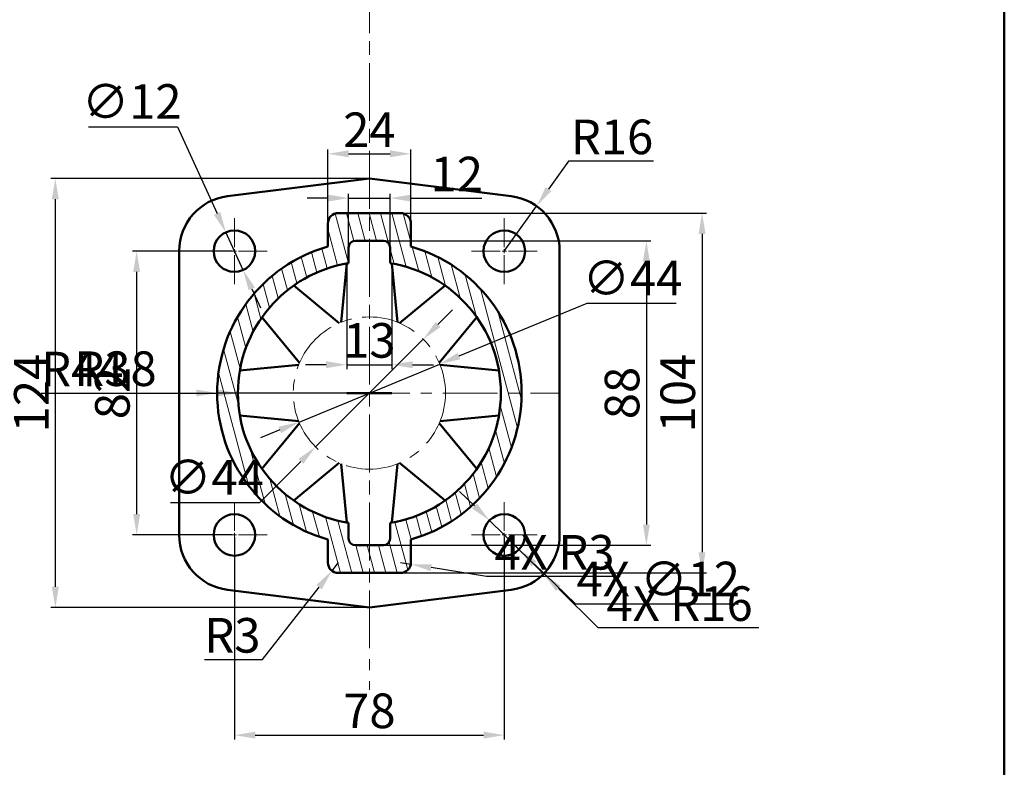
# Model space of a CAD drawing. Units: millimetres. Extents: x 147 to 984, y -369 to 435.
# Tile 9 of 10: x 699 to 984, y -34 to 182. Entities that reach past the tile are written whole.
import ezdxf

# ---------------------------------------------------------------- set-up
doc = ezdxf.new("R2010")
doc.units = ezdxf.units.MM
doc.header["$LTSCALE"] = 0.5
doc.linetypes.add('CENTER', pattern=[50.8, 31.75, -6.35, 6.35, -6.35])
for name, color, linetype, lineweight in [('M-CNTR', 1, 'CENTER', 18), ('M-DIMS', 2, 'Continuous', 25), ('M-HATC', 8, 'Continuous', 18), ('M-OUTL', 7, 'Continuous', 50)]:
    doc.layers.add(name, color=color, linetype=linetype, lineweight=lineweight)
doc.styles.get("Standard").update_dxf_attribs({"font": 'arial.ttf'})
doc.dimstyles.new('ISO-25', dxfattribs={"dimtxt": 10, "dimasz": 6, "dimexe": 1.25, "dimexo": 0.625, "dimtad": 1, "dimtoh": 1, "dimdec": 0, "dimtxsty": 'Standard', "dimcen": 2.5, "dimadec": 0, "dimazin": 0, "dimtfac": 1, "dimtdec": 0, "dimtmove": 0, "dimatfit": 3, "dimfxl": 1, "dimarcsym": 0})

# ---------------------------------------------------------------- blocks, each defined once
blk = doc.blocks.new('*U58')
at = {"layer": 'M-CNTR', "color": 0, "transparency": 16777216}
for p, q in [((0, 1.2), (0, 9.5)), ((-9.5, 0), (-1.2, 0)), ((1.2, 0), (9.5, 0)), ((0, -9.5), (0, -1.2))]:
    blk.add_line(p, q, dxfattribs=at)
at = {"layer": 'M-CNTR', "color": 0, "linetype": 'Continuous', "transparency": 16777216}
for p, q in [((-0.6, 0), (0.6, 0)), ((0, -0.6), (0, 0.6))]:
    blk.add_line(p, q, dxfattribs=at)
blk = doc.blocks.new('*U59')
at = {"layer": 'M-CNTR', "color": 0, "transparency": 16777216}
for p, q in [((0, 1.2), (0, 9.5)), ((-9.5, 0), (-1.2, 0)), ((1.2, 0), (9.5, 0)), ((0, -9.5), (0, -1.2))]:
    blk.add_line(p, q, dxfattribs=at)
at = {"layer": 'M-CNTR', "color": 0, "linetype": 'Continuous', "transparency": 16777216}
for p, q in [((-0.6, 0), (0.6, 0)), ((0, -0.6), (0, 0.6))]:
    blk.add_line(p, q, dxfattribs=at)
blk = doc.blocks.new('*U60')
at = {"layer": 'M-CNTR', "color": 0, "transparency": 16777216}
for p, q in [((0, 1.2), (0, 9.5)), ((-9.5, 0), (-1.2, 0)), ((1.2, 0), (9.5, 0)), ((0, -9.5), (0, -1.2))]:
    blk.add_line(p, q, dxfattribs=at)
at = {"layer": 'M-CNTR', "color": 0, "linetype": 'Continuous', "transparency": 16777216}
for p, q in [((-0.6, 0), (0.6, 0)), ((0, -0.6), (0, 0.6))]:
    blk.add_line(p, q, dxfattribs=at)
blk = doc.blocks.new('*U61')
at = {"layer": 'M-CNTR', "color": 0, "transparency": 16777216}
for p, q in [((0, 1.2), (0, 9.5)), ((-9.5, 0), (-1.2, 0)), ((1.2, 0), (9.5, 0)), ((0, -9.5), (0, -1.2))]:
    blk.add_line(p, q, dxfattribs=at)
at = {"layer": 'M-CNTR', "color": 0, "linetype": 'Continuous', "transparency": 16777216}
for p, q in [((-0.6, 0), (0.6, 0)), ((0, -0.6), (0, 0.6))]:
    blk.add_line(p, q, dxfattribs=at)
blk = doc.blocks.new('*U62')
at = {"layer": 'M-CNTR', "color": 0, "transparency": 16777216}
blk.add_line((0, 99.41), (0, -106.28), dxfattribs=at)
blk = doc.blocks.new('*D63')
at = {"layer": 'Defpoints', "color": 0, "transparency": 16777216}
for p in [(800.56, 136.03), (709.78, 12.03), (800.56, 12.03)]:
    blk.add_point(p, dxfattribs=at)
at = {"layer": 'M-DIMS', "color": 0, "lineweight": -2, "transparency": 16777216}
for p, q in [((799.93, 136.03), (708.53, 136.03)), ((709.78, 130.03), (709.78, 18.03)), ((799.93, 12.03), (708.53, 12.03))]:
    blk.add_line(p, q, dxfattribs=at)
at = {"layer": 'M-DIMS', "color": 0, "transparency": 16777216}
for points in [[(708.78, 130.03), (710.78, 130.03), (709.78, 136.03)], [(708.78, 18.03), (710.78, 18.03), (709.78, 12.03)]]:
    blk.add_solid(points, dxfattribs=at)
at = {"layer": 'M-DIMS', "color": 0, "transparency": 16777216, "insert": (704.14, 74.03), "char_height": 10, "attachment_point": 5, "rotation": 90}
blk.add_mtext('124', dxfattribs=at)
blk = doc.blocks.new('*D64')
at = {"layer": 'Defpoints', "color": 0, "transparency": 16777216}
for p in [(761.56, 115.03), (733.29, 33.03), (761.56, 33.03)]:
    blk.add_point(p, dxfattribs=at)
at = {"layer": 'M-DIMS', "color": 0, "lineweight": -2, "transparency": 16777216}
for p, q in [((760.93, 115.03), (732.04, 115.03)), ((733.29, 109.03), (733.29, 39.03)), ((760.93, 33.03), (732.04, 33.03))]:
    blk.add_line(p, q, dxfattribs=at)
at = {"layer": 'M-DIMS', "color": 0, "transparency": 16777216}
for points in [[(732.29, 109.03), (734.29, 109.03), (733.29, 115.03)], [(732.29, 39.03), (734.29, 39.03), (733.29, 33.03)]]:
    blk.add_solid(points, dxfattribs=at)
at = {"layer": 'M-DIMS', "color": 0, "transparency": 16777216, "insert": (727.56, 74.03), "char_height": 10, "attachment_point": 5, "rotation": 90}
blk.add_mtext('82', dxfattribs=at)
blk = doc.blocks.new('*D65')
at = {"layer": 'Defpoints', "color": 0, "transparency": 16777216}
for p in [(759.05, 120.48), (764.06, 109.58)]:
    blk.add_point(p, dxfattribs=at)
at = {"layer": 'M-DIMS', "color": 0, "lineweight": -2, "transparency": 16777216}
for p, q in [((719.33, 150.97), (745.06, 150.97)), ((745.06, 150.97), (756.55, 125.93)), ((764.06, 109.58), (759.05, 120.48)), ((766.56, 104.12), (769.07, 98.67))]:
    blk.add_line(p, q, dxfattribs=at)
at = {"layer": 'M-DIMS', "color": 0, "transparency": 16777216}
for points in [[(757.46, 126.35), (755.64, 125.52), (759.05, 120.48)], [(767.47, 104.54), (765.66, 103.7), (764.06, 109.58)]]:
    blk.add_solid(points, dxfattribs=at)
at = {"layer": 'M-DIMS', "color": 0, "transparency": 16777216, "insert": (731.88, 156.98), "char_height": 10, "attachment_point": 5}
blk.add_mtext('∅12', dxfattribs=at)
blk = doc.blocks.new('*D66')
at = {"layer": 'Defpoints', "color": 0, "transparency": 16777216}
for p in [(848.86, 128.04), (839.56, 115.03)]:
    blk.add_point(p, dxfattribs=at)
at = {"layer": 'M-DIMS', "color": 0, "lineweight": -2, "transparency": 16777216}
for p, q in [((858.14, 141.02), (852.35, 132.92)), ((882.65, 141.02), (858.14, 141.02)), ((839.56, 115.03), (848.86, 128.04))]:
    blk.add_line(p, q, dxfattribs=at)
at = {"layer": 'M-DIMS', "color": 0, "transparency": 16777216}
blk.add_solid([(851.54, 133.51), (853.17, 132.34), (848.86, 128.04)], dxfattribs=at)
at = {"layer": 'M-DIMS', "color": 0, "transparency": 16777216, "insert": (870.71, 146.75), "char_height": 10, "attachment_point": 5}
blk.add_mtext('R16', dxfattribs=at)
blk = doc.blocks.new('*D67')
at = {"layer": 'Defpoints', "color": 0, "transparency": 16777216}
for p in [(812.56, 143.16), (788.56, 119.69), (812.56, 119.69)]:
    blk.add_point(p, dxfattribs=at)
at = {"layer": 'M-DIMS', "color": 0, "lineweight": -2, "transparency": 16777216}
for p, q in [((788.56, 120.32), (788.56, 144.41)), ((794.56, 143.16), (806.56, 143.16)), ((812.56, 120.32), (812.56, 144.41))]:
    blk.add_line(p, q, dxfattribs=at)
at = {"layer": 'M-DIMS', "color": 0, "transparency": 16777216}
for points in [[(794.56, 144.16), (794.56, 142.16), (788.56, 143.16)], [(806.56, 144.16), (806.56, 142.16), (812.56, 143.16)]]:
    blk.add_solid(points, dxfattribs=at)
at = {"layer": 'M-DIMS', "color": 0, "transparency": 16777216, "insert": (800.56, 148.8), "char_height": 10, "attachment_point": 5}
blk.add_mtext('24', dxfattribs=at)
blk = doc.blocks.new('*D68')
at = {"layer": 'Defpoints', "color": 0, "transparency": 16777216}
for p in [(806.56, 130.37), (794.56, 113.79), (806.56, 113.79)]:
    blk.add_point(p, dxfattribs=at)
at = {"layer": 'M-DIMS', "color": 0, "lineweight": -2, "transparency": 16777216}
for p, q in [((794.56, 114.41), (794.56, 131.62)), ((806.56, 114.41), (806.56, 131.62)), ((788.56, 130.37), (782.56, 130.37)), ((794.56, 130.37), (806.56, 130.37)), ((812.56, 130.37), (833.09, 130.37))]:
    blk.add_line(p, q, dxfattribs=at)
at = {"layer": 'M-DIMS', "color": 0, "transparency": 16777216}
for points in [[(788.56, 131.37), (788.56, 129.37), (794.56, 130.37)], [(812.56, 131.37), (812.56, 129.37), (806.56, 130.37)]]:
    blk.add_solid(points, dxfattribs=at)
at = {"layer": 'M-DIMS', "color": 0, "transparency": 16777216, "insert": (825.82, 136.01), "char_height": 10, "attachment_point": 5}
blk.add_mtext('12', dxfattribs=at)
blk = doc.blocks.new('*D69')
at = {"layer": 'Defpoints', "color": 0, "transparency": 16777216}
for p in [(794.06, 111.47), (807.06, 111.47), (807.06, 82.22)]:
    blk.add_point(p, dxfattribs=at)
at = {"layer": 'M-DIMS', "color": 0, "lineweight": -2, "transparency": 16777216}
for p, q in [((794.06, 110.84), (794.06, 80.97)), ((807.06, 110.84), (807.06, 80.97)), ((788.06, 82.22), (782.06, 82.22)), ((794.06, 82.22), (807.06, 82.22)), ((813.06, 82.22), (819.06, 82.22))]:
    blk.add_line(p, q, dxfattribs=at)
at = {"layer": 'M-DIMS', "color": 0, "transparency": 16777216}
for points in [[(788.06, 83.22), (788.06, 81.22), (794.06, 82.22)], [(813.06, 83.22), (813.06, 81.22), (807.06, 82.22)]]:
    blk.add_solid(points, dxfattribs=at)
at = {"layer": 'M-DIMS', "color": 0, "transparency": 16777216, "insert": (800.56, 87.95), "char_height": 10, "attachment_point": 5}
blk.add_mtext('13', dxfattribs=at)
blk = doc.blocks.new('*D70')
at = {"layer": 'Defpoints', "color": 0, "transparency": 16777216}
for p in [(820.9, 82.41), (780.22, 65.64)]:
    blk.add_point(p, dxfattribs=at)
at = {"layer": 'M-DIMS', "color": 0, "lineweight": -2, "transparency": 16777216}
for p, q in [((863.42, 99.94), (826.44, 84.7)), ((889.21, 99.94), (863.42, 99.94)), ((780.22, 65.64), (820.9, 82.41)), ((774.67, 63.36), (769.12, 61.07))]:
    blk.add_line(p, q, dxfattribs=at)
at = {"layer": 'M-DIMS', "color": 0, "transparency": 16777216}
for points in [[(826.06, 85.62), (826.83, 83.77), (820.9, 82.41)], [(774.29, 64.28), (775.05, 62.43), (780.22, 65.64)]]:
    blk.add_solid(points, dxfattribs=at)
at = {"layer": 'M-DIMS', "color": 0, "transparency": 16777216, "insert": (876.63, 105.95), "char_height": 10, "attachment_point": 5}
blk.add_mtext('∅44', dxfattribs=at)
blk = doc.blocks.new('*D71')
at = {"layer": 'Defpoints', "color": 0, "transparency": 16777216}
for p in [(800.56, 126.03), (800.56, 22.03), (896.72, 22.03)]:
    blk.add_point(p, dxfattribs=at)
at = {"layer": 'M-DIMS', "color": 0, "lineweight": -2, "transparency": 16777216}
for p, q in [((801.18, 126.03), (897.97, 126.03)), ((896.72, 120.03), (896.72, 28.03)), ((801.18, 22.03), (897.97, 22.03))]:
    blk.add_line(p, q, dxfattribs=at)
at = {"layer": 'M-DIMS', "color": 0, "transparency": 16777216}
for points in [[(895.72, 120.03), (897.72, 120.03), (896.72, 126.03)], [(895.72, 28.03), (897.72, 28.03), (896.72, 22.03)]]:
    blk.add_solid(points, dxfattribs=at)
at = {"layer": 'M-DIMS', "color": 0, "transparency": 16777216, "insert": (890.99, 74.03), "char_height": 10, "attachment_point": 5, "rotation": 90}
blk.add_mtext('104', dxfattribs=at)
blk = doc.blocks.new('*D72')
at = {"layer": 'Defpoints', "color": 0, "transparency": 16777216}
for p in [(791.56, 25.03), (789.71, 22.66)]:
    blk.add_point(p, dxfattribs=at)
at = {"layer": 'M-DIMS', "color": 0, "lineweight": -2, "transparency": 16777216}
for p, q in [((791.56, 25.03), (789.71, 22.66)), ((769.66, -3.02), (786.02, 17.93)), ((752.91, -3.02), (769.66, -3.02))]:
    blk.add_line(p, q, dxfattribs=at)
at = {"layer": 'M-DIMS', "color": 0, "transparency": 16777216}
blk.add_solid([(785.23, 18.55), (786.81, 17.32), (789.71, 22.66)], dxfattribs=at)
at = {"layer": 'M-DIMS', "color": 0, "transparency": 16777216, "insert": (760.97, 2.72), "char_height": 10, "attachment_point": 5}
blk.add_mtext('R3', dxfattribs=at)
blk = doc.blocks.new('*D73')
at = {"layer": 'Defpoints', "color": 0, "transparency": 16777216}
for p in [(761.56, 33.03), (839.56, 33.03), (839.56, -24.83)]:
    blk.add_point(p, dxfattribs=at)
at = {"layer": 'M-DIMS', "color": 0, "lineweight": -2, "transparency": 16777216}
for p, q in [((761.56, 32.4), (761.56, -26.08)), ((839.56, 32.4), (839.56, -26.08)), ((767.56, -24.83), (833.56, -24.83))]:
    blk.add_line(p, q, dxfattribs=at)
at = {"layer": 'M-DIMS', "color": 0, "transparency": 16777216}
for points in [[(767.56, -23.83), (767.56, -25.83), (761.56, -24.83)], [(833.56, -23.83), (833.56, -25.83), (839.56, -24.83)]]:
    blk.add_solid(points, dxfattribs=at)
at = {"layer": 'M-DIMS', "color": 0, "transparency": 16777216, "insert": (800.56, -19.1), "char_height": 10, "attachment_point": 5}
blk.add_mtext('78', dxfattribs=at)
blk = doc.blocks.new('*D74')
at = {"layer": 'Defpoints', "color": 0, "transparency": 16777216}
for p in [(800.56, 118.03), (800.56, 30.03), (880.62, 30.03)]:
    blk.add_point(p, dxfattribs=at)
at = {"layer": 'M-DIMS', "color": 0, "lineweight": -2, "transparency": 16777216}
for p, q in [((801.18, 118.03), (881.87, 118.03)), ((880.62, 112.03), (880.62, 36.03)), ((801.18, 30.03), (881.87, 30.03))]:
    blk.add_line(p, q, dxfattribs=at)
at = {"layer": 'M-DIMS', "color": 0, "transparency": 16777216}
for points in [[(879.62, 112.03), (881.62, 112.03), (880.62, 118.03)], [(879.62, 36.03), (881.62, 36.03), (880.62, 30.03)]]:
    blk.add_solid(points, dxfattribs=at)
at = {"layer": 'M-DIMS', "color": 0, "transparency": 16777216, "insert": (874.89, 74.03), "char_height": 10, "attachment_point": 5, "rotation": 90}
blk.add_mtext('88', dxfattribs=at)
blk = doc.blocks.new('*D174')
at = {"layer": 'Defpoints', "color": 0, "ltscale": 0.5, "transparency": 16777216}
for p in [(756.56, 74.03), (800.56, 74.03)]:
    blk.add_point(p, dxfattribs=at)
at = {"layer": 'M-DIMS', "color": 0, "lineweight": -2, "ltscale": 0.5, "transparency": 16777216}
for p, q in [((705.68, 74.03), (730.16, 74.03)), ((730.16, 74.03), (750.56, 74.03)), ((800.56, 74.03), (756.56, 74.03))]:
    blk.add_line(p, q, dxfattribs=at)
at = {"layer": 'M-DIMS', "color": 0, "ltscale": 0.5, "transparency": 16777216}
blk.add_solid([(750.56, 75.03), (750.56, 73.03), (756.56, 74.03)], dxfattribs=at)
at = {"layer": 'M-DIMS', "color": 0, "ltscale": 0.5, "transparency": 16777216, "insert": (717.61, 79.65), "char_height": 10, "attachment_point": 5}
blk.add_mtext('R44', dxfattribs=at)
blk = doc.blocks.new('*D175')
at = {"layer": 'Defpoints', "color": 0, "ltscale": 0.5, "transparency": 16777216}
for p in [(762.56, 74.03), (800.56, 74.03)]:
    blk.add_point(p, dxfattribs=at)
at = {"layer": 'M-DIMS', "color": 0, "lineweight": -2, "ltscale": 0.5, "transparency": 16777216}
for p, q in [((715.22, 74.03), (739.76, 74.03)), ((739.76, 74.03), (756.56, 74.03)), ((800.56, 74.03), (762.56, 74.03))]:
    blk.add_line(p, q, dxfattribs=at)
at = {"layer": 'M-DIMS', "color": 0, "ltscale": 0.5, "transparency": 16777216}
blk.add_solid([(756.56, 75.03), (756.56, 73.03), (762.56, 74.03)], dxfattribs=at)
at = {"layer": 'M-DIMS', "color": 0, "ltscale": 0.5, "transparency": 16777216, "insert": (727.17, 79.76), "char_height": 10, "attachment_point": 5}
blk.add_mtext('R38', dxfattribs=at)
blk = doc.blocks.new('*D176')
at = {"layer": 'Defpoints', "color": 0, "ltscale": 0.5, "transparency": 16777216}
for p in [(816.13, 89.57), (784.99, 58.49)]:
    blk.add_point(p, dxfattribs=at)
at = {"layer": 'M-DIMS', "color": 0, "lineweight": -2, "ltscale": 0.5, "transparency": 16777216}
for p, q in [((820.38, 93.81), (824.62, 98.05)), ((816.13, 89.57), (784.99, 58.49)), ((768.87, 42.4), (780.74, 54.25)), ((743.08, 42.4), (768.87, 42.4))]:
    blk.add_line(p, q, dxfattribs=at)
at = {"layer": 'M-DIMS', "color": 0, "ltscale": 0.5, "transparency": 16777216}
for points in [[(819.67, 94.52), (821.08, 93.1), (816.13, 89.57)], [(780.03, 54.96), (781.45, 53.54), (784.99, 58.49)]]:
    blk.add_solid(points, dxfattribs=at)
at = {"layer": 'M-DIMS', "color": 0, "ltscale": 0.5, "transparency": 16777216, "insert": (755.66, 48.41), "char_height": 10, "attachment_point": 5}
blk.add_mtext('∅44', dxfattribs=at)
blk = doc.blocks.new('*D177')
at = {"layer": 'Defpoints', "color": 0, "ltscale": 0.5, "transparency": 16777216}
for p in [(835.25, 37.21), (843.86, 28.85)]:
    blk.add_point(p, dxfattribs=at)
at = {"layer": 'M-DIMS', "color": 0, "lineweight": -2, "ltscale": 0.5, "transparency": 16777216}
for p, q in [((830.95, 41.39), (826.65, 45.57)), ((835.25, 37.21), (843.86, 28.85)), ((860.19, 12.98), (848.16, 24.67)), ((907.28, 12.98), (860.19, 12.98))]:
    blk.add_line(p, q, dxfattribs=at)
at = {"layer": 'M-DIMS', "color": 0, "ltscale": 0.5, "transparency": 16777216}
for points in [[(831.65, 42.11), (830.25, 40.67), (835.25, 37.21)], [(848.86, 25.38), (847.47, 23.95), (843.86, 28.85)]]:
    blk.add_solid(points, dxfattribs=at)
at = {"layer": 'M-DIMS', "color": 0, "ltscale": 0.5, "transparency": 16777216, "insert": (884.05, 18.99), "char_height": 10, "attachment_point": 5}
blk.add_mtext('4X ∅12', dxfattribs=at)
blk = doc.blocks.new('*D178')
at = {"layer": 'Defpoints', "color": 0, "ltscale": 0.5, "transparency": 16777216}
for p in [(839.56, 33.03), (850.93, 21.77)]:
    blk.add_point(p, dxfattribs=at)
at = {"layer": 'M-DIMS', "color": 0, "lineweight": -2, "ltscale": 0.5, "transparency": 16777216}
for p, q in [((839.56, 33.03), (850.93, 21.77)), ((866.72, 6.15), (855.19, 17.55)), ((913.12, 6.15), (866.72, 6.15))]:
    blk.add_line(p, q, dxfattribs=at)
at = {"layer": 'M-DIMS', "color": 0, "ltscale": 0.5, "transparency": 16777216}
blk.add_solid([(855.9, 18.26), (854.49, 16.84), (850.93, 21.77)], dxfattribs=at)
at = {"layer": 'M-DIMS', "color": 0, "ltscale": 0.5, "transparency": 16777216, "insert": (890.23, 11.88), "char_height": 10, "attachment_point": 5}
blk.add_mtext('4X R16', dxfattribs=at)
blk = doc.blocks.new('*D179')
at = {"layer": 'Defpoints', "color": 0, "ltscale": 0.5, "transparency": 16777216}
for p in [(809.56, 25.03), (812.52, 24.55)]:
    blk.add_point(p, dxfattribs=at)
at = {"layer": 'M-DIMS', "color": 0, "lineweight": -2, "ltscale": 0.5, "transparency": 16777216}
for p, q in [((809.56, 25.03), (812.52, 24.55)), ((834.45, 20.98), (818.44, 23.58)), ((873.09, 20.98), (834.45, 20.98))]:
    blk.add_line(p, q, dxfattribs=at)
at = {"layer": 'M-DIMS', "color": 0, "ltscale": 0.5, "transparency": 16777216}
blk.add_solid([(818.6, 24.57), (818.28, 22.59), (812.52, 24.55)], dxfattribs=at)
at = {"layer": 'M-DIMS', "color": 0, "ltscale": 0.5, "transparency": 16777216, "insert": (854.08, 26.71), "char_height": 10, "attachment_point": 5}
blk.add_mtext('4X R3', dxfattribs=at)

msp = doc.modelspace()

# ---------------------------------------------------------------- hatches: boundary and pattern name
at = {"layer": 'M-HATC'}
h = msp.add_hatch(dxfattribs=at)
h.set_pattern_fill('ANSI31', color=256, angle=60)
h.set_pattern_definition([(105, (-593.0547, -70.8474), (-3.0668145, -0.8217505), [])])
h.paths.add_polyline_path([(762.5575, 74.0279), (756.5575, 74.0279, 0.33543674), (788.5575, 31.6959), (788.5575, 25.0279, 0.41421356), (791.5575, 22.0279), (800.5575, 22.0279), (800.5575, 30.0279), (796.5575, 30.0279, -0.41421356), (794.5575, 32.0279), (794.5575, 36.5046, -0.36849956)])
h.paths.add_polyline_path([(794.5575, 111.5512), (794.5575, 116.0279, -0.41421356), (796.5575, 118.0279), (804.5575, 118.0279, -0.41421356), (806.5575, 116.0279), (806.5575, 111.5512, -0.36849956), (838.5575, 74.0279), (844.5575, 74.0279, 0.33543674), (812.5575, 116.3599), (812.5575, 123.0279, 0.41421356), (809.5575, 126.0279), (791.5575, 126.0279, 0.41421356), (788.5575, 123.0279), (788.5575, 116.3599, 0.33543674), (756.5575, 74.0279), (762.5575, 74.0279, -0.36849956)])
h.paths.add_polyline_path([(844.5575, 74.0279), (838.5575, 74.0279, -0.36849956), (806.5575, 36.5046), (806.5575, 32.0279, -0.41421356), (804.5575, 30.0279), (800.5575, 30.0279), (800.5575, 22.0279), (809.5575, 22.0279, 0.41421356), (812.5575, 25.0279), (812.5575, 31.6959, 0.33543674)])

# ---------------------------------------------------------------- linework, layer by layer
at = {"layer": 'M-CNTR'}
for p, q in [((800.5575, 321.7953), (800.5575, 4.2226)), ((745.5575, 74.0279), (855.5575, 74.0279))]:
    msp.add_line(p, q, dxfattribs=at)
msp.add_circle((800.5575, 74.0279), 22, dxfattribs=at)
at = {"layer": 'M-OUTL'}
for p, q in [((759.5727, 130.9043), (800.5575, 136.0279)), ((800.5575, 136.0279), (841.5422, 130.9043)), ((809.5575, 126.0279), (791.5575, 126.0279)), ((788.5575, 116.3599), (788.5575, 123.0279)), ((812.5575, 116.3599), (812.5575, 123.0279)), ((745.5575, 115.0279), (745.5575, 74.0279)), ((855.5575, 74.0279), (855.5575, 115.0279)), ((792.4053, 94.4618), (794.0575, 111.4679)), ((808.7096, 94.4618), (807.0575, 111.4679)), ((791.873, 94.2413), (778.6796, 105.0982)), ((809.242, 94.2413), (822.4353, 105.0982)), ((780.3441, 82.7124), (769.4873, 95.9058)), ((820.7708, 82.7124), (831.6277, 95.9058)), ((780.1236, 82.1801), (763.1175, 80.5279)), ((820.9913, 82.1801), (837.9974, 80.5279)), ((745.5575, 74.0279), (745.5575, 33.0279)), ((794.0575, 74.0279), (807.0575, 74.0279)), ((855.5575, 33.0279), (855.5575, 74.0279)), ((780.1236, 65.8758), (763.1175, 67.5279)), ((820.9913, 65.8758), (837.9974, 67.5279)), ((780.3441, 65.3434), (769.4873, 52.1501)), ((820.7708, 65.3434), (831.6277, 52.1501)), ((791.873, 53.8146), (778.6796, 42.9577)), ((792.4053, 53.5941), (794.0575, 36.588)), ((808.7096, 53.5941), (807.0575, 36.588)), ((809.242, 53.8146), (822.4353, 42.9577)), ((788.5575, 31.6959), (788.5575, 25.0279)), ((812.5575, 31.6959), (812.5575, 25.0279)), ((809.5575, 22.0279), (791.5575, 22.0279)), ((759.5727, 17.1515), (800.5575, 12.0279)), ((800.5575, 12.0279), (841.5422, 17.1515))]:
    msp.add_line(p, q, dxfattribs=at)
at = {"layer": 'M-OUTL', "ltscale": 0.5}
msp.add_lwpolyline([(147.3511, 435.3078), (984.0884, 435.3078), (984.0884, -369.4968), (147.3511, -369.4968)], close=True, dxfattribs=at)
at = {"layer": 'M-OUTL'}
for points in [[(794.5575, 111.5512), (794.5575, 116.0279, -0.41421356), (796.5575, 118.0279), (804.5575, 118.0279, -0.41421356), (806.5575, 116.0279), (806.5575, 111.5512)], [(806.5575, 36.5046), (806.5575, 32.0279, -0.41421356), (804.5575, 30.0279), (796.5575, 30.0279, -0.41421356), (794.5575, 32.0279), (794.5575, 36.5046)]]:
    msp.add_lwpolyline(points, format="xyb", dxfattribs=at)
for centre in [(761.5575, 115.0279), (839.5575, 115.0279), (761.5575, 33.0279), (839.5575, 33.0279)]:
    msp.add_circle(centre, 6, dxfattribs=at)
for centre, radius, start, end in [((761.5575, 115.0279), 16, 97.125683, 180), ((839.5575, 115.0279), 16, 0, 82.874317), ((791.5575, 123.0279), 3, 90, 180), ((809.5575, 123.0279), 3, 0, 90), ((800.5575, 74.0279), 44, 105.82662, 254.17338), ((800.5575, 74.0279), 44, 285.82662, 74.17338), ((800.5575, 74.0279), 38, 99.08472, 260.91528), ((800.5575, 74.0279), 38, 279.08472, 80.91528), ((761.5575, 33.0279), 16, 180, 262.874317), ((839.5575, 33.0279), 16, 277.125683, 0), ((791.5575, 25.0279), 3, 180, 270), ((809.5575, 25.0279), 3, 270, 0)]:
    msp.add_arc(centre, radius, start, end, dxfattribs=at)

# ---------------------------------------------------------------- block references
at = {"layer": 'M-CNTR'}
for name, p in [('*U62', (800.5575, 94.5279)), ('*U59', (761.5575, 115.0279)), ('*U58', (839.5575, 115.0279)), ('*U61', (761.5575, 33.0279)), ('*U60', (839.5575, 33.0279))]:
    msp.add_blockref(name, p, dxfattribs=at)

# ---------------------------------------------------------------- dimensions: what is measured, and where the dimension line sits
at = {"layer": 'M-DIMS'}
for p1, p2, picture, middle in [((764.0607, 109.5751), (759.0542, 120.4808), '*D65', (731.8797, 150.9736)), ((780.2178, 65.6436), (820.8972, 82.4123), '*D70', (876.6289, 99.9417))]:
    dim = msp.add_diameter_dim_2p(p1=p1, p2=p2, dimstyle='ISO-25', override={"dimclrd": 0, "dimclre": 0, "dimclrt": 0}, dxfattribs=at)
    dim.commit()
    dim.dimension.update_dxf_attribs({"geometry": picture, "text_midpoint": middle, "dimtype": 163})
for base, p1, p2, picture, middle in [((812.5575, 143.1557), (788.5575, 119.6939), (812.5575, 119.6939), '*D67', (800.5575, 148.8011)), ((806.5575, 130.3657), (794.5575, 113.7896), (806.5575, 113.7896), '*D68', (825.823, 136.0111)), ((839.5575, -24.8274), (761.5575, 33.0279), (839.5575, 33.0279), '*D73', (800.5575, -19.0967))]:
    dim = msp.add_linear_dim(base=base, p1=p1, p2=p2, dimstyle='ISO-25', override={"dimclrd": 0, "dimclre": 0, "dimclrt": 0}, dxfattribs=at)
    dim.commit()
    dim.dimension.update_dxf_attribs({"geometry": picture, "text_midpoint": middle})
for center, mpoint, picture, middle in [((839.5575, 115.0279), (848.8631, 128.0435), '*D66', (870.7072, 141.0162)), ((791.5575, 25.0279), (789.7111, 22.6634), '*D72', (760.9703, -3.0177))]:
    dim = msp.add_radius_dim(center=center, mpoint=mpoint, dimstyle='ISO-25', override={"dimclrd": 0, "dimclre": 0, "dimclrt": 0}, dxfattribs=at)
    dim.commit()
    dim.dimension.update_dxf_attribs({"geometry": picture, "text_midpoint": middle, "dimtype": 164})
for base, p1, p2, picture, middle in [((709.7842, 12.0279), (800.5575, 136.0279), (800.5575, 12.0279), '*D63', (704.1387, 74.0279)), ((896.7231, 22.0279), (800.5575, 126.0279), (800.5575, 22.0279), '*D71', (890.9924, 74.0279)), ((880.62, 30.0279), (800.5575, 118.0279), (800.5575, 30.0279), '*D74', (874.8893, 74.0279)), ((733.287, 33.0279), (761.5575, 115.0279), (761.5575, 33.0279), '*D64', (727.5563, 74.0279))]:
    dim = msp.add_linear_dim(base=base, p1=p1, p2=p2, angle=90, dimstyle='ISO-25', override={"dimclrd": 0, "dimclre": 0, "dimclrt": 0}, dxfattribs=at)
    dim.commit()
    dim.dimension.update_dxf_attribs({"geometry": picture, "text_midpoint": middle})
dim = msp.add_linear_dim(base=(807.0575, 82.2171), p1=(794.0575, 111.4679), p2=(807.0575, 111.4679), dimstyle='ISO-25', override={"dimclrd": 0, "dimclre": 0, "dimclrt": 0}, dxfattribs=at)
dim.commit()
dim.dimension.update_dxf_attribs({"geometry": '*D69', "text_midpoint": (800.5575, 82.2171), "dimtype": 160})
at = {"layer": 'M-DIMS', "ltscale": 0.5}
dim = msp.add_diameter_dim_2p(p1=(816.1286, 89.5695), p2=(784.9863, 58.4864), dimstyle='ISO-25', override={"dimdec": 0, "dimlfac": 1, "dimrnd": 0, "dimzin": 0, "dimdsep": 46, "dimlunit": 2}, dxfattribs=at)
dim.commit()
dim.dimension.update_dxf_attribs({"geometry": '*D176', "text_midpoint": (755.6628, 42.4003), "dimtype": 163})
for mpoint, picture, middle in [((756.5575, 74.028), '*D174', (730.1575, 74.0281)), ((762.5575, 74.028), '*D175', (739.7575, 74.0281))]:
    dim = msp.add_radius_dim(center=(800.5575, 74.0279), mpoint=mpoint, dimstyle='ISO-25', override={"dimdec": 0, "dimlfac": 1, "dimrnd": 0, "dimzin": 0, "dimdsep": 46, "dimlunit": 2}, dxfattribs=at)
    dim.commit()
    dim.dimension.update_dxf_attribs({"geometry": picture, "text_midpoint": middle, "dimtype": 164})
dim = msp.add_diameter_dim_2p(p1=(835.2543, 37.2091), p2=(843.8607, 28.8467), text='4X <>', dimstyle='ISO-25', override={"dimdec": 0, "dimlfac": 1, "dimrnd": 0, "dimzin": 0, "dimdsep": 46, "dimlunit": 2}, dxfattribs=at)
dim.commit()
dim.dimension.update_dxf_attribs({"geometry": '*D177', "text_midpoint": (884.0468, 12.9785), "dimtype": 163})
for center, mpoint, picture, middle in [((809.5575, 25.0279), (812.5185, 24.5458), '*D179', (854.0805, 26.7096)), ((839.5575, 33.0279), (850.9295, 21.7728), '*D178', (890.2302, 11.8791))]:
    dim = msp.add_radius_dim(center=center, mpoint=mpoint, text='4X <>', dimstyle='ISO-25', override={"dimdec": 0, "dimlfac": 1, "dimrnd": 0, "dimzin": 0, "dimdsep": 46, "dimlunit": 2}, dxfattribs=at)
    dim.commit()
    dim.dimension.update_dxf_attribs({"geometry": picture, "text_midpoint": middle})

doc.saveas('drawing.dxf')
